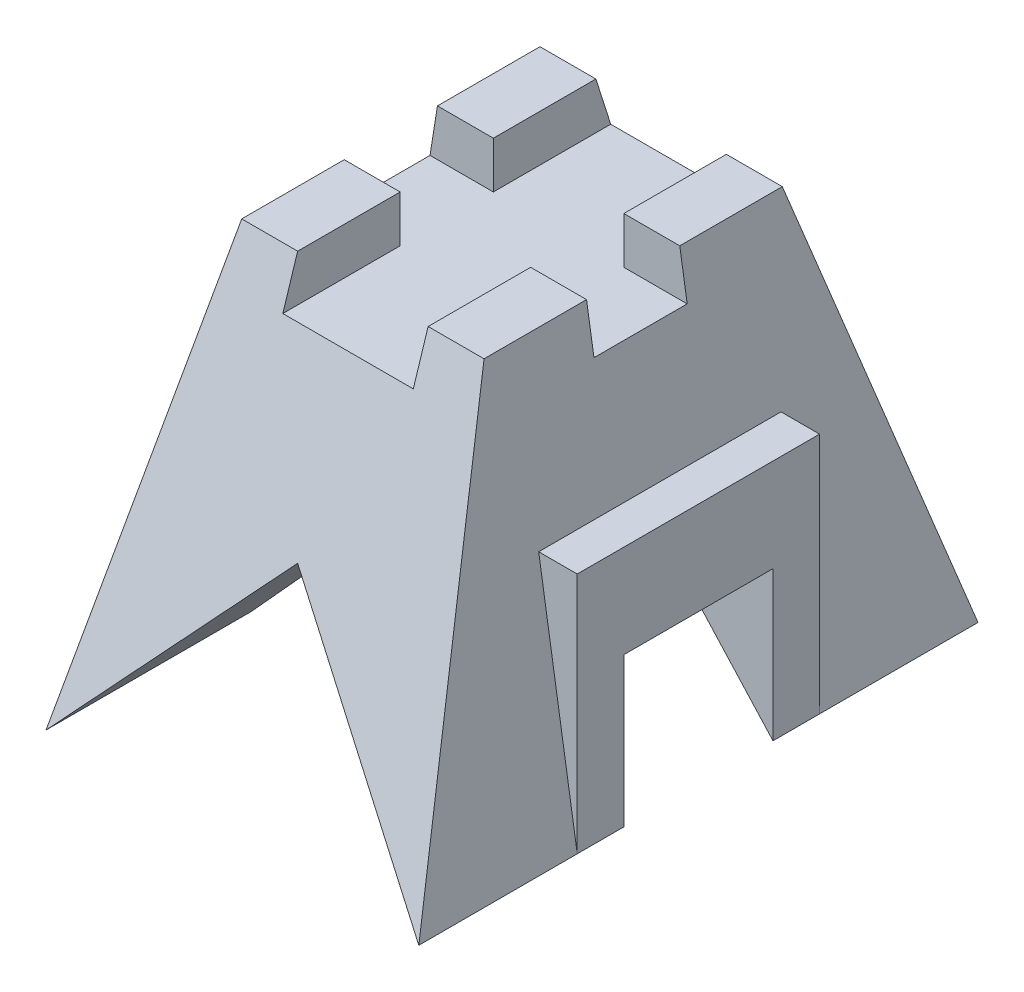
ISO-10303-21;
HEADER;
FILE_DESCRIPTION(('STEP AP214'),'2;1');
FILE_NAME('part.step','',(''),(''),'','','');
FILE_SCHEMA(('AUTOMOTIVE_DESIGN { 1 0 10303 214 1 1 1 1 }'));
ENDSEC;
DATA;
#1=APPLICATION_CONTEXT('core data for automotive mechanical design processes');
#2=APPLICATION_PROTOCOL_DEFINITION('international standard','automotive_design',2000,#1);
#3=PRODUCT_CONTEXT('',#1,'mechanical');
#4=PRODUCT('Part','Part','',(#3));
#5=PRODUCT_RELATED_PRODUCT_CATEGORY('part','',(#4));
#6=PRODUCT_DEFINITION_FORMATION('','',#4);
#7=PRODUCT_DEFINITION_CONTEXT('part definition',#1,'design');
#8=PRODUCT_DEFINITION('design','',#6,#7);
#9=PRODUCT_DEFINITION_SHAPE('','',#8);
#10=(LENGTH_UNIT() NAMED_UNIT(*) SI_UNIT(.MILLI.,.METRE.));
#11=(NAMED_UNIT(*) PLANE_ANGLE_UNIT() SI_UNIT($,.RADIAN.));
#12=(NAMED_UNIT(*) SI_UNIT($,.STERADIAN.) SOLID_ANGLE_UNIT());
#13=UNCERTAINTY_MEASURE_WITH_UNIT(LENGTH_MEASURE(1.E-05),#10,'distance_accuracy_value','');
#14=(GEOMETRIC_REPRESENTATION_CONTEXT(3) GLOBAL_UNCERTAINTY_ASSIGNED_CONTEXT((#13)) GLOBAL_UNIT_ASSIGNED_CONTEXT((#10,
#11,#12)) REPRESENTATION_CONTEXT('',''));
#15=CARTESIAN_POINT('',(0.,0.,0.));
#16=DIRECTION('',(0.,0.,1.));
#17=DIRECTION('',(1.,0.,0.));
#18=AXIS2_PLACEMENT_3D('',#15,#16,#17);
#19=CARTESIAN_POINT('',(100.,0.,65.));
#20=DIRECTION('',(-1.,0.,0.));
#21=DIRECTION('',(0.,0.,1.));
#22=AXIS2_PLACEMENT_3D('',#19,#20,#21);
#23=PLANE('',#22);
#24=DIRECTION('',(0.,-1.,0.));
#25=VECTOR('',#24,1.);
#26=CARTESIAN_POINT('',(100.,0.,40.));
#27=LINE('',#26,#25);
#28=CARTESIAN_POINT('',(100.,80.,40.));
#29=VERTEX_POINT('',#28);
#30=CARTESIAN_POINT('',(100.,0.,40.));
#31=VERTEX_POINT('',#30);
#32=EDGE_CURVE('E103',#29,#31,#27,.T.);
#33=ORIENTED_EDGE('',*,*,#32,.F.);
#34=DIRECTION('',(0.,0.,1.));
#35=VECTOR('',#34,1.);
#36=CARTESIAN_POINT('',(100.,80.,40.));
#37=LINE('',#36,#35);
#38=CARTESIAN_POINT('',(100.,80.,-40.));
#39=VERTEX_POINT('',#38);
#40=EDGE_CURVE('E99',#39,#29,#37,.T.);
#41=ORIENTED_EDGE('',*,*,#40,.F.);
#42=DIRECTION('',(0.,1.,0.));
#43=VECTOR('',#42,1.);
#44=CARTESIAN_POINT('',(100.,0.,-40.));
#45=LINE('',#44,#43);
#46=CARTESIAN_POINT('',(100.,0.,-40.));
#47=VERTEX_POINT('',#46);
#48=EDGE_CURVE('E89',#47,#39,#45,.T.);
#49=ORIENTED_EDGE('',*,*,#48,.F.);
#50=DIRECTION('',(0.,0.,1.));
#51=VECTOR('',#50,1.);
#52=CARTESIAN_POINT('',(100.,0.,65.));
#53=LINE('',#52,#51);
#54=CARTESIAN_POINT('',(100.,0.,-65.));
#55=VERTEX_POINT('',#54);
#56=EDGE_CURVE('E46',#47,#55,#53,.F.);
#57=ORIENTED_EDGE('',*,*,#56,.T.);
#58=DIRECTION('',(0.,1.,0.));
#59=VECTOR('',#58,1.);
#60=CARTESIAN_POINT('',(100.,0.,-65.));
#61=LINE('',#60,#59);
#62=CARTESIAN_POINT('',(100.,130.,-65.));
#63=VERTEX_POINT('',#62);
#64=EDGE_CURVE('E260',#55,#63,#61,.T.);
#65=ORIENTED_EDGE('',*,*,#64,.T.);
#66=DIRECTION('',(0.,0.,-1.));
#67=VECTOR('',#66,1.);
#68=CARTESIAN_POINT('',(100.,130.,65.));
#69=LINE('',#68,#67);
#70=CARTESIAN_POINT('',(100.,130.,65.));
#71=VERTEX_POINT('',#70);
#72=EDGE_CURVE('E107',#71,#63,#69,.T.);
#73=ORIENTED_EDGE('',*,*,#72,.F.);
#74=DIRECTION('',(0.,1.,0.));
#75=VECTOR('',#74,1.);
#76=CARTESIAN_POINT('',(100.,0.,65.));
#77=LINE('',#76,#75);
#78=CARTESIAN_POINT('',(100.,0.,65.));
#79=VERTEX_POINT('',#78);
#80=EDGE_CURVE('E249',#79,#71,#77,.T.);
#81=ORIENTED_EDGE('',*,*,#80,.F.);
#82=DIRECTION('',(0.,0.,1.));
#83=VECTOR('',#82,1.);
#84=CARTESIAN_POINT('',(100.,0.,65.));
#85=LINE('',#84,#83);
#86=EDGE_CURVE('E108',#79,#31,#85,.F.);
#87=ORIENTED_EDGE('',*,*,#86,.T.);
#88=EDGE_LOOP('',(#33,#41,#49,#57,#65,#73,#81,#87));
#89=FACE_BOUND('',#88,.T.);
#90=ADVANCED_FACE('F45',(#89),#23,.F.);
#91=CARTESIAN_POINT('',(-100.,0.,65.));
#92=DIRECTION('',(-1.,0.,0.));
#93=DIRECTION('',(0.,0.,1.));
#94=AXIS2_PLACEMENT_3D('',#91,#92,#93);
#95=PLANE('',#94);
#96=DIRECTION('',(0.,0.,1.));
#97=VECTOR('',#96,1.);
#98=CARTESIAN_POINT('',(-100.,80.,40.));
#99=LINE('',#98,#97);
#100=CARTESIAN_POINT('',(-100.,80.,-40.));
#101=VERTEX_POINT('',#100);
#102=CARTESIAN_POINT('',(-100.,80.,40.));
#103=VERTEX_POINT('',#102);
#104=EDGE_CURVE('E781',#101,#103,#99,.T.);
#105=ORIENTED_EDGE('',*,*,#104,.T.);
#106=DIRECTION('',(0.,-1.,0.));
#107=VECTOR('',#106,1.);
#108=CARTESIAN_POINT('',(-100.,0.,40.));
#109=LINE('',#108,#107);
#110=CARTESIAN_POINT('',(-100.,0.,40.));
#111=VERTEX_POINT('',#110);
#112=EDGE_CURVE('E265',#103,#111,#109,.T.);
#113=ORIENTED_EDGE('',*,*,#112,.T.);
#114=DIRECTION('',(0.,0.,-1.));
#115=VECTOR('',#114,1.);
#116=CARTESIAN_POINT('',(-100.,0.,65.));
#117=LINE('',#116,#115);
#118=CARTESIAN_POINT('',(-100.,0.,65.));
#119=VERTEX_POINT('',#118);
#120=EDGE_CURVE('E393',#119,#111,#117,.T.);
#121=ORIENTED_EDGE('',*,*,#120,.F.);
#122=DIRECTION('',(0.,1.,0.));
#123=VECTOR('',#122,1.);
#124=CARTESIAN_POINT('',(-100.,0.,65.));
#125=LINE('',#124,#123);
#126=CARTESIAN_POINT('',(-100.,130.,65.));
#127=VERTEX_POINT('',#126);
#128=EDGE_CURVE('E378',#119,#127,#125,.T.);
#129=ORIENTED_EDGE('',*,*,#128,.T.);
#130=DIRECTION('',(0.,0.,-1.));
#131=VECTOR('',#130,1.);
#132=CARTESIAN_POINT('',(-100.,130.,65.));
#133=LINE('',#132,#131);
#134=CARTESIAN_POINT('',(-100.,130.,-65.));
#135=VERTEX_POINT('',#134);
#136=EDGE_CURVE('E399',#127,#135,#133,.T.);
#137=ORIENTED_EDGE('',*,*,#136,.T.);
#138=DIRECTION('',(0.,1.,0.));
#139=VECTOR('',#138,1.);
#140=CARTESIAN_POINT('',(-100.,0.,-65.));
#141=LINE('',#140,#139);
#142=CARTESIAN_POINT('',(-100.,0.,-65.));
#143=VERTEX_POINT('',#142);
#144=EDGE_CURVE('E409',#143,#135,#141,.T.);
#145=ORIENTED_EDGE('',*,*,#144,.F.);
#146=CARTESIAN_POINT('',(-100.,0.,-40.));
#147=VERTEX_POINT('',#146);
#148=EDGE_CURVE('E388',#147,#143,#117,.T.);
#149=ORIENTED_EDGE('',*,*,#148,.F.);
#150=DIRECTION('',(0.,1.,0.));
#151=VECTOR('',#150,1.);
#152=CARTESIAN_POINT('',(-100.,0.,-40.));
#153=LINE('',#152,#151);
#154=EDGE_CURVE('E788',#147,#101,#153,.T.);
#155=ORIENTED_EDGE('',*,*,#154,.T.);
#156=EDGE_LOOP('',(#105,#113,#121,#129,#137,#145,#149,#155));
#157=FACE_BOUND('',#156,.T.);
#158=ADVANCED_FACE('F398',(#157),#95,.T.);
#159=CARTESIAN_POINT('',(65.,220.,-150.));
#160=DIRECTION('',(0.987580306335114,0.157115048735132,0.));
#161=DIRECTION('',(-0.157115048735132,0.987580306335114,0.));
#162=AXIS2_PLACEMENT_3D('',#159,#160,#161);
#163=PLANE('',#162);
#164=DIRECTION('',(0.,0.,-1.));
#165=VECTOR('',#164,1.);
#166=CARTESIAN_POINT('',(79.3181818181818,130.,65.));
#167=LINE('',#166,#165);
#168=CARTESIAN_POINT('',(79.3181818181818,130.,65.));
#169=VERTEX_POINT('',#168);
#170=CARTESIAN_POINT('',(79.3181818181818,130.,-65.));
#171=VERTEX_POINT('',#170);
#172=EDGE_CURVE('E113',#169,#171,#167,.T.);
#173=ORIENTED_EDGE('',*,*,#172,.T.);
#174=DIRECTION('',(0.157115048735132,-0.987580306335114,0.));
#175=VECTOR('',#174,1.);
#176=CARTESIAN_POINT('',(79.3181818181818,130.,-65.));
#177=LINE('',#176,#175);
#178=EDGE_CURVE('E256',#171,#55,#177,.T.);
#179=ORIENTED_EDGE('',*,*,#178,.T.);
#180=DIRECTION('',(0.,0.,-1.));
#181=VECTOR('',#180,1.);
#182=CARTESIAN_POINT('',(100.,0.,-150.));
#183=LINE('',#182,#181);
#184=CARTESIAN_POINT('',(100.,0.,-150.));
#185=VERTEX_POINT('',#184);
#186=EDGE_CURVE('E110',#55,#185,#183,.T.);
#187=ORIENTED_EDGE('',*,*,#186,.T.);
#188=DIRECTION('',(-0.149889153602658,0.942160394073851,0.299778307205316));
#189=VECTOR('',#188,1.);
#190=CARTESIAN_POINT('',(65.7863365428702,215.057313159101,-81.5726730857405));
#191=LINE('',#190,#189);
#192=CARTESIAN_POINT('',(65.,220.,-80.));
#193=VERTEX_POINT('',#192);
#194=EDGE_CURVE('E168',#185,#193,#191,.T.);
#195=ORIENTED_EDGE('',*,*,#194,.T.);
#196=DIRECTION('',(0.,0.,1.));
#197=VECTOR('',#196,1.);
#198=CARTESIAN_POINT('',(65.,220.,-150.));
#199=LINE('',#198,#197);
#200=CARTESIAN_POINT('',(65.,220.,-25.));
#201=VERTEX_POINT('',#200);
#202=EDGE_CURVE('E153',#193,#201,#199,.T.);
#203=ORIENTED_EDGE('',*,*,#202,.T.);
#204=DIRECTION('',(0.157115048735132,-0.987580306335114,0.));
#205=VECTOR('',#204,1.);
#206=CARTESIAN_POINT('',(65.8639798488665,214.569269521411,-25.));
#207=LINE('',#206,#205);
#208=CARTESIAN_POINT('',(68.9772727272727,195.,-25.));
#209=VERTEX_POINT('',#208);
#210=EDGE_CURVE('E161',#201,#209,#207,.T.);
#211=ORIENTED_EDGE('',*,*,#210,.T.);
#212=DIRECTION('',(0.,0.,1.));
#213=VECTOR('',#212,1.);
#214=CARTESIAN_POINT('',(68.9772727272727,195.,25.));
#215=LINE('',#214,#213);
#216=CARTESIAN_POINT('',(68.9772727272727,195.,25.));
#217=VERTEX_POINT('',#216);
#218=EDGE_CURVE('E157',#209,#217,#215,.T.);
#219=ORIENTED_EDGE('',*,*,#218,.T.);
#220=DIRECTION('',(-0.157115048735132,0.987580306335114,0.));
#221=VECTOR('',#220,1.);
#222=CARTESIAN_POINT('',(65.8639798488665,214.569269521411,25.));
#223=LINE('',#222,#221);
#224=CARTESIAN_POINT('',(65.,220.,25.));
#225=VERTEX_POINT('',#224);
#226=EDGE_CURVE('E160',#217,#225,#223,.T.);
#227=ORIENTED_EDGE('',*,*,#226,.T.);
#228=CARTESIAN_POINT('',(65.,220.,80.));
#229=VERTEX_POINT('',#228);
#230=EDGE_CURVE('E135',#225,#229,#199,.T.);
#231=ORIENTED_EDGE('',*,*,#230,.T.);
#232=DIRECTION('',(0.149889153602658,-0.942160394073851,0.299778307205316));
#233=VECTOR('',#232,1.);
#234=CARTESIAN_POINT('',(100.,0.,150.));
#235=LINE('',#234,#233);
#236=CARTESIAN_POINT('',(100.,0.,150.));
#237=VERTEX_POINT('',#236);
#238=EDGE_CURVE('E231',#229,#237,#235,.T.);
#239=ORIENTED_EDGE('',*,*,#238,.T.);
#240=EDGE_CURVE('E201',#237,#79,#183,.T.);
#241=ORIENTED_EDGE('',*,*,#240,.T.);
#242=DIRECTION('',(0.157115048735132,-0.987580306335114,0.));
#243=VECTOR('',#242,1.);
#244=CARTESIAN_POINT('',(79.3181818181818,130.,65.));
#245=LINE('',#244,#243);
#246=EDGE_CURVE('E254',#169,#79,#245,.T.);
#247=ORIENTED_EDGE('',*,*,#246,.F.);
#248=EDGE_LOOP('',(#173,#179,#187,#195,#203,#211,#219,#227,#231,#239,#241,#247));
#249=FACE_BOUND('',#248,.T.);
#250=ADVANCED_FACE('F288',(#249),#163,.T.);
#251=CARTESIAN_POINT('',(100.,220.,-25.));
#252=DIRECTION('',(0.,-1.,0.));
#253=DIRECTION('',(0.,0.,-1.));
#254=AXIS2_PLACEMENT_3D('',#251,#252,#253);
#255=PLANE('',#254);
#256=DIRECTION('',(0.,0.,1.));
#257=VECTOR('',#256,1.);
#258=CARTESIAN_POINT('',(-35.,220.,-150.));
#259=LINE('',#258,#257);
#260=CARTESIAN_POINT('',(-35.,220.,-80.));
#261=VERTEX_POINT('',#260);
#262=CARTESIAN_POINT('',(-35.,220.,-25.));
#263=VERTEX_POINT('',#262);
#264=EDGE_CURVE('E136',#261,#263,#259,.T.);
#265=ORIENTED_EDGE('',*,*,#264,.F.);
#266=DIRECTION('',(-1.,0.,0.));
#267=VECTOR('',#266,1.);
#268=CARTESIAN_POINT('',(100.,220.,-80.));
#269=LINE('',#268,#267);
#270=CARTESIAN_POINT('',(-65.,220.,-80.));
#271=VERTEX_POINT('',#270);
#272=EDGE_CURVE('E230',#261,#271,#269,.T.);
#273=ORIENTED_EDGE('',*,*,#272,.T.);
#274=DIRECTION('',(0.,0.,1.));
#275=VECTOR('',#274,1.);
#276=CARTESIAN_POINT('',(-65.,220.,-150.));
#277=LINE('',#276,#275);
#278=CARTESIAN_POINT('',(-65.,220.,-25.));
#279=VERTEX_POINT('',#278);
#280=EDGE_CURVE('E140',#271,#279,#277,.T.);
#281=ORIENTED_EDGE('',*,*,#280,.T.);
#282=DIRECTION('',(-1.,0.,0.));
#283=VECTOR('',#282,1.);
#284=CARTESIAN_POINT('',(100.,220.,-25.));
#285=LINE('',#284,#283);
#286=EDGE_CURVE('E222',#263,#279,#285,.T.);
#287=ORIENTED_EDGE('',*,*,#286,.F.);
#288=EDGE_LOOP('',(#265,#273,#281,#287));
#289=FACE_BOUND('',#288,.T.);
#290=ADVANCED_FACE('F445',(#289),#255,.F.);
#291=ORIENTED_EDGE('',*,*,#202,.F.);
#292=CARTESIAN_POINT('',(35.,220.,-80.));
#293=VERTEX_POINT('',#292);
#294=EDGE_CURVE('E235',#193,#293,#269,.T.);
#295=ORIENTED_EDGE('',*,*,#294,.T.);
#296=DIRECTION('',(0.,0.,1.));
#297=VECTOR('',#296,1.);
#298=CARTESIAN_POINT('',(35.,220.,-150.));
#299=LINE('',#298,#297);
#300=CARTESIAN_POINT('',(35.,220.,-25.));
#301=VERTEX_POINT('',#300);
#302=EDGE_CURVE('E148',#293,#301,#299,.T.);
#303=ORIENTED_EDGE('',*,*,#302,.T.);
#304=EDGE_CURVE('E226',#201,#301,#285,.T.);
#305=ORIENTED_EDGE('',*,*,#304,.F.);
#306=EDGE_LOOP('',(#291,#295,#303,#305));
#307=FACE_BOUND('',#306,.T.);
#308=ADVANCED_FACE('F542',(#307),#255,.F.);
#309=CARTESIAN_POINT('',(100.,220.,80.));
#310=DIRECTION('',(0.,-1.,0.));
#311=DIRECTION('',(0.,0.,-1.));
#312=AXIS2_PLACEMENT_3D('',#309,#310,#311);
#313=PLANE('',#312);
#314=CARTESIAN_POINT('',(-35.,220.,25.));
#315=VERTEX_POINT('',#314);
#316=CARTESIAN_POINT('',(-35.,220.,79.9999999999999));
#317=VERTEX_POINT('',#316);
#318=EDGE_CURVE('E139',#315,#317,#259,.T.);
#319=ORIENTED_EDGE('',*,*,#318,.F.);
#320=DIRECTION('',(-1.,0.,0.));
#321=VECTOR('',#320,1.);
#322=CARTESIAN_POINT('',(100.,220.,25.));
#323=LINE('',#322,#321);
#324=CARTESIAN_POINT('',(-65.,220.,25.));
#325=VERTEX_POINT('',#324);
#326=EDGE_CURVE('E214',#315,#325,#323,.T.);
#327=ORIENTED_EDGE('',*,*,#326,.T.);
#328=CARTESIAN_POINT('',(-65.,220.,80.));
#329=VERTEX_POINT('',#328);
#330=EDGE_CURVE('E133',#325,#329,#277,.T.);
#331=ORIENTED_EDGE('',*,*,#330,.T.);
#332=DIRECTION('',(-1.,0.,0.));
#333=VECTOR('',#332,1.);
#334=CARTESIAN_POINT('',(100.,220.,80.));
#335=LINE('',#334,#333);
#336=EDGE_CURVE('E207',#317,#329,#335,.T.);
#337=ORIENTED_EDGE('',*,*,#336,.F.);
#338=EDGE_LOOP('',(#319,#327,#331,#337));
#339=FACE_BOUND('',#338,.T.);
#340=ADVANCED_FACE('F417',(#339),#313,.F.);
#341=ORIENTED_EDGE('',*,*,#230,.F.);
#342=CARTESIAN_POINT('',(35.,220.,25.));
#343=VERTEX_POINT('',#342);
#344=EDGE_CURVE('E219',#225,#343,#323,.T.);
#345=ORIENTED_EDGE('',*,*,#344,.T.);
#346=CARTESIAN_POINT('',(35.,220.,80.));
#347=VERTEX_POINT('',#346);
#348=EDGE_CURVE('E154',#343,#347,#299,.T.);
#349=ORIENTED_EDGE('',*,*,#348,.T.);
#350=EDGE_CURVE('E215',#229,#347,#335,.T.);
#351=ORIENTED_EDGE('',*,*,#350,.F.);
#352=EDGE_LOOP('',(#341,#345,#349,#351));
#353=FACE_BOUND('',#352,.T.);
#354=ADVANCED_FACE('F543',(#353),#313,.F.);
#355=CARTESIAN_POINT('',(100.,220.,-80.));
#356=DIRECTION('',(0.,-0.303203657276947,0.952925780013262));
#357=DIRECTION('',(0.,-0.952925780013262,-0.303203657276947));
#358=AXIS2_PLACEMENT_3D('',#355,#356,#357);
#359=PLANE('',#358);
#360=DIRECTION('',(-0.654770604471651,0.720247664918816,0.229169711565078));
#361=VECTOR('',#360,1.);
#362=CARTESIAN_POINT('',(-14.2550911039657,125.680600214362,-110.010718113612));
#363=LINE('',#362,#361);
#364=CARTESIAN_POINT('',(0.,110.,-115.));
#365=VERTEX_POINT('',#364);
#366=EDGE_CURVE('E130',#185,#365,#363,.T.);
#367=ORIENTED_EDGE('',*,*,#366,.T.);
#368=DIRECTION('',(-0.654770604471651,-0.720247664918816,-0.229169711565078));
#369=VECTOR('',#368,1.);
#370=CARTESIAN_POINT('',(100.,220.,-80.));
#371=LINE('',#370,#369);
#372=CARTESIAN_POINT('',(-100.,0.,-150.));
#373=VERTEX_POINT('',#372);
#374=EDGE_CURVE('E128',#365,#373,#371,.T.);
#375=ORIENTED_EDGE('',*,*,#374,.T.);
#376=DIRECTION('',(-0.149889153602658,-0.942160394073851,-0.299778307205316));
#377=VECTOR('',#376,1.);
#378=CARTESIAN_POINT('',(-61.292984869326,243.301237964237,-72.585969738652));
#379=LINE('',#378,#377);
#380=EDGE_CURVE('E198',#271,#373,#379,.T.);
#381=ORIENTED_EDGE('',*,*,#380,.F.);
#382=ORIENTED_EDGE('',*,*,#272,.F.);
#383=DIRECTION('',(0.,0.952925780013262,0.303203657276947));
#384=VECTOR('',#383,1.);
#385=CARTESIAN_POINT('',(-35.,220.,-80.));
#386=LINE('',#385,#384);
#387=CARTESIAN_POINT('',(-35.,195.,-87.9545454545455));
#388=VERTEX_POINT('',#387);
#389=EDGE_CURVE('E190',#388,#261,#386,.T.);
#390=ORIENTED_EDGE('',*,*,#389,.F.);
#391=DIRECTION('',(-1.,0.,0.));
#392=VECTOR('',#391,1.);
#393=CARTESIAN_POINT('',(100.,195.,-87.9545454545455));
#394=LINE('',#393,#392);
#395=CARTESIAN_POINT('',(35.,195.,-87.9545454545455));
#396=VERTEX_POINT('',#395);
#397=EDGE_CURVE('E178',#396,#388,#394,.T.);
#398=ORIENTED_EDGE('',*,*,#397,.F.);
#399=DIRECTION('',(0.,-0.952925780013262,-0.303203657276947));
#400=VECTOR('',#399,1.);
#401=CARTESIAN_POINT('',(35.,220.,-80.));
#402=LINE('',#401,#400);
#403=EDGE_CURVE('E174',#293,#396,#402,.T.);
#404=ORIENTED_EDGE('',*,*,#403,.F.);
#405=ORIENTED_EDGE('',*,*,#294,.F.);
#406=ORIENTED_EDGE('',*,*,#194,.F.);
#407=EDGE_LOOP('',(#367,#375,#381,#382,#390,#398,#404,#405,#406));
#408=FACE_BOUND('',#407,.T.);
#409=ADVANCED_FACE('F42',(#408),#359,.F.);
#410=CARTESIAN_POINT('',(100.,220.,-25.));
#411=DIRECTION('',(0.,0.,-1.));
#412=DIRECTION('',(0.,1.,0.));
#413=AXIS2_PLACEMENT_3D('',#410,#411,#412);
#414=PLANE('',#413);
#415=DIRECTION('',(0.157115048735132,0.987580306335114,0.));
#416=VECTOR('',#415,1.);
#417=CARTESIAN_POINT('',(-60.926952141058,245.60201511335,-25.));
#418=LINE('',#417,#416);
#419=CARTESIAN_POINT('',(-68.9772727272727,195.,-25.));
#420=VERTEX_POINT('',#419);
#421=EDGE_CURVE('E199',#420,#279,#418,.T.);
#422=ORIENTED_EDGE('',*,*,#421,.F.);
#423=DIRECTION('',(-1.,0.,0.));
#424=VECTOR('',#423,1.);
#425=CARTESIAN_POINT('',(100.,195.,-25.));
#426=LINE('',#425,#424);
#427=CARTESIAN_POINT('',(-35.,195.,-25.));
#428=VERTEX_POINT('',#427);
#429=EDGE_CURVE('E223',#428,#420,#426,.T.);
#430=ORIENTED_EDGE('',*,*,#429,.F.);
#431=DIRECTION('',(0.,-1.,0.));
#432=VECTOR('',#431,1.);
#433=CARTESIAN_POINT('',(-35.,220.,-25.));
#434=LINE('',#433,#432);
#435=EDGE_CURVE('E183',#263,#428,#434,.T.);
#436=ORIENTED_EDGE('',*,*,#435,.F.);
#437=ORIENTED_EDGE('',*,*,#286,.T.);
#438=EDGE_LOOP('',(#422,#430,#436,#437));
#439=FACE_BOUND('',#438,.T.);
#440=ADVANCED_FACE('F436',(#439),#414,.F.);
#441=DIRECTION('',(0.,1.,0.));
#442=VECTOR('',#441,1.);
#443=CARTESIAN_POINT('',(35.,220.,-25.));
#444=LINE('',#443,#442);
#445=CARTESIAN_POINT('',(35.,195.,-25.));
#446=VERTEX_POINT('',#445);
#447=EDGE_CURVE('E175',#446,#301,#444,.T.);
#448=ORIENTED_EDGE('',*,*,#447,.F.);
#449=EDGE_CURVE('E224',#209,#446,#426,.T.);
#450=ORIENTED_EDGE('',*,*,#449,.F.);
#451=ORIENTED_EDGE('',*,*,#210,.F.);
#452=ORIENTED_EDGE('',*,*,#304,.T.);
#453=EDGE_LOOP('',(#448,#450,#451,#452));
#454=FACE_BOUND('',#453,.T.);
#455=ADVANCED_FACE('F547',(#454),#414,.F.);
#456=CARTESIAN_POINT('',(100.,195.,25.));
#457=DIRECTION('',(0.,-1.,0.));
#458=DIRECTION('',(0.,0.,-1.));
#459=AXIS2_PLACEMENT_3D('',#456,#457,#458);
#460=PLANE('',#459);
#461=ORIENTED_EDGE('',*,*,#449,.T.);
#462=DIRECTION('',(0.,0.,1.));
#463=VECTOR('',#462,1.);
#464=CARTESIAN_POINT('',(35.,195.,-150.));
#465=LINE('',#464,#463);
#466=EDGE_CURVE('E147',#396,#446,#465,.T.);
#467=ORIENTED_EDGE('',*,*,#466,.F.);
#468=ORIENTED_EDGE('',*,*,#397,.T.);
#469=DIRECTION('',(0.,0.,1.));
#470=VECTOR('',#469,1.);
#471=CARTESIAN_POINT('',(-35.,195.,-150.));
#472=LINE('',#471,#470);
#473=EDGE_CURVE('E145',#388,#428,#472,.T.);
#474=ORIENTED_EDGE('',*,*,#473,.T.);
#475=ORIENTED_EDGE('',*,*,#429,.T.);
#476=DIRECTION('',(0.,0.,-1.));
#477=VECTOR('',#476,1.);
#478=CARTESIAN_POINT('',(-68.9772727272727,195.,25.));
#479=LINE('',#478,#477);
#480=CARTESIAN_POINT('',(-68.9772727272727,195.,25.));
#481=VERTEX_POINT('',#480);
#482=EDGE_CURVE('E194',#481,#420,#479,.T.);
#483=ORIENTED_EDGE('',*,*,#482,.F.);
#484=DIRECTION('',(-1.,0.,0.));
#485=VECTOR('',#484,1.);
#486=CARTESIAN_POINT('',(100.,195.,25.));
#487=LINE('',#486,#485);
#488=CARTESIAN_POINT('',(-35.,195.,25.));
#489=VERTEX_POINT('',#488);
#490=EDGE_CURVE('E216',#489,#481,#487,.T.);
#491=ORIENTED_EDGE('',*,*,#490,.F.);
#492=CARTESIAN_POINT('',(-35.,195.,87.9545454545455));
#493=VERTEX_POINT('',#492);
#494=EDGE_CURVE('E141',#489,#493,#472,.T.);
#495=ORIENTED_EDGE('',*,*,#494,.T.);
#496=DIRECTION('',(1.,0.,0.));
#497=VECTOR('',#496,1.);
#498=CARTESIAN_POINT('',(100.,195.,87.9545454545455));
#499=LINE('',#498,#497);
#500=CARTESIAN_POINT('',(35.,195.,87.9545454545455));
#501=VERTEX_POINT('',#500);
#502=EDGE_CURVE('E237',#493,#501,#499,.T.);
#503=ORIENTED_EDGE('',*,*,#502,.T.);
#504=CARTESIAN_POINT('',(35.,195.,25.));
#505=VERTEX_POINT('',#504);
#506=EDGE_CURVE('E150',#505,#501,#465,.T.);
#507=ORIENTED_EDGE('',*,*,#506,.F.);
#508=EDGE_CURVE('E217',#217,#505,#487,.T.);
#509=ORIENTED_EDGE('',*,*,#508,.F.);
#510=ORIENTED_EDGE('',*,*,#218,.F.);
#511=EDGE_LOOP('',(#461,#467,#468,#474,#475,#483,#491,#495,#503,#507,#509,#510));
#512=FACE_BOUND('',#511,.T.);
#513=ADVANCED_FACE('F427',(#512),#460,.F.);
#514=CARTESIAN_POINT('',(100.,220.,25.));
#515=DIRECTION('',(0.,0.,1.));
#516=DIRECTION('',(0.,-1.,0.));
#517=AXIS2_PLACEMENT_3D('',#514,#515,#516);
#518=PLANE('',#517);
#519=DIRECTION('',(-0.157115048735132,-0.987580306335114,0.));
#520=VECTOR('',#519,1.);
#521=CARTESIAN_POINT('',(-60.926952141058,245.60201511335,25.));
#522=LINE('',#521,#520);
#523=EDGE_CURVE('E188',#325,#481,#522,.T.);
#524=ORIENTED_EDGE('',*,*,#523,.F.);
#525=ORIENTED_EDGE('',*,*,#326,.F.);
#526=DIRECTION('',(0.,1.,0.));
#527=VECTOR('',#526,1.);
#528=CARTESIAN_POINT('',(-35.,220.,25.));
#529=LINE('',#528,#527);
#530=EDGE_CURVE('E181',#489,#315,#529,.T.);
#531=ORIENTED_EDGE('',*,*,#530,.F.);
#532=ORIENTED_EDGE('',*,*,#490,.T.);
#533=EDGE_LOOP('',(#524,#525,#531,#532));
#534=FACE_BOUND('',#533,.T.);
#535=ADVANCED_FACE('F425',(#534),#518,.F.);
#536=DIRECTION('',(0.,-1.,0.));
#537=VECTOR('',#536,1.);
#538=CARTESIAN_POINT('',(35.,220.,25.));
#539=LINE('',#538,#537);
#540=EDGE_CURVE('E169',#343,#505,#539,.T.);
#541=ORIENTED_EDGE('',*,*,#540,.F.);
#542=ORIENTED_EDGE('',*,*,#344,.F.);
#543=ORIENTED_EDGE('',*,*,#226,.F.);
#544=ORIENTED_EDGE('',*,*,#508,.T.);
#545=EDGE_LOOP('',(#541,#542,#543,#544));
#546=FACE_BOUND('',#545,.T.);
#547=ADVANCED_FACE('F544',(#546),#518,.F.);
#548=CARTESIAN_POINT('',(100.,0.,150.));
#549=DIRECTION('',(0.,-0.303203657276947,-0.952925780013262));
#550=DIRECTION('',(0.,0.952925780013262,-0.303203657276947));
#551=AXIS2_PLACEMENT_3D('',#548,#549,#550);
#552=PLANE('',#551);
#553=DIRECTION('',(0.149889153602658,0.942160394073851,-0.299778307205316));
#554=VECTOR('',#553,1.);
#555=CARTESIAN_POINT('',(-95.5066483264557,28.2439248051352,141.013296652912));
#556=LINE('',#555,#554);
#557=CARTESIAN_POINT('',(-100.,0.,150.));
#558=VERTEX_POINT('',#557);
#559=EDGE_CURVE('E244',#558,#329,#556,.T.);
#560=ORIENTED_EDGE('',*,*,#559,.F.);
#561=DIRECTION('',(0.654770604471651,0.720247664918816,-0.229169711565078));
#562=VECTOR('',#561,1.);
#563=CARTESIAN_POINT('',(-14.2550911039657,94.3193997856377,119.989281886388));
#564=LINE('',#563,#562);
#565=CARTESIAN_POINT('',(0.,110.,115.));
#566=VERTEX_POINT('',#565);
#567=EDGE_CURVE('E12',#558,#566,#564,.T.);
#568=ORIENTED_EDGE('',*,*,#567,.T.);
#569=DIRECTION('',(0.654770604471651,-0.720247664918816,0.229169711565078));
#570=VECTOR('',#569,1.);
#571=CARTESIAN_POINT('',(100.,0.,150.));
#572=LINE('',#571,#570);
#573=EDGE_CURVE('E55',#566,#237,#572,.T.);
#574=ORIENTED_EDGE('',*,*,#573,.T.);
#575=ORIENTED_EDGE('',*,*,#238,.F.);
#576=ORIENTED_EDGE('',*,*,#350,.T.);
#577=DIRECTION('',(0.,0.952925780013262,-0.303203657276947));
#578=VECTOR('',#577,1.);
#579=CARTESIAN_POINT('',(35.,0.,150.));
#580=LINE('',#579,#578);
#581=EDGE_CURVE('E236',#501,#347,#580,.T.);
#582=ORIENTED_EDGE('',*,*,#581,.F.);
#583=ORIENTED_EDGE('',*,*,#502,.F.);
#584=DIRECTION('',(0.,-0.952925780013262,0.303203657276947));
#585=VECTOR('',#584,1.);
#586=CARTESIAN_POINT('',(-35.,0.,150.));
#587=LINE('',#586,#585);
#588=EDGE_CURVE('E245',#317,#493,#587,.T.);
#589=ORIENTED_EDGE('',*,*,#588,.F.);
#590=ORIENTED_EDGE('',*,*,#336,.T.);
#591=EDGE_LOOP('',(#560,#568,#574,#575,#576,#582,#583,#589,#590));
#592=FACE_BOUND('',#591,.T.);
#593=ADVANCED_FACE('F415',(#592),#552,.F.);
#594=CARTESIAN_POINT('',(35.,220.,-150.));
#595=DIRECTION('',(-1.,0.,0.));
#596=DIRECTION('',(0.,-1.,0.));
#597=AXIS2_PLACEMENT_3D('',#594,#595,#596);
#598=PLANE('',#597);
#599=ORIENTED_EDGE('',*,*,#540,.T.);
#600=ORIENTED_EDGE('',*,*,#506,.T.);
#601=ORIENTED_EDGE('',*,*,#581,.T.);
#602=ORIENTED_EDGE('',*,*,#348,.F.);
#603=EDGE_LOOP('',(#599,#600,#601,#602));
#604=FACE_BOUND('',#603,.T.);
#605=ADVANCED_FACE('F537',(#604),#598,.T.);
#606=CARTESIAN_POINT('',(-35.,220.,-150.));
#607=DIRECTION('',(1.,0.,0.));
#608=DIRECTION('',(0.,1.,0.));
#609=AXIS2_PLACEMENT_3D('',#606,#607,#608);
#610=PLANE('',#609);
#611=ORIENTED_EDGE('',*,*,#530,.T.);
#612=ORIENTED_EDGE('',*,*,#318,.T.);
#613=ORIENTED_EDGE('',*,*,#588,.T.);
#614=ORIENTED_EDGE('',*,*,#494,.F.);
#615=EDGE_LOOP('',(#611,#612,#613,#614));
#616=FACE_BOUND('',#615,.T.);
#617=ADVANCED_FACE('F529',(#616),#610,.T.);
#618=CARTESIAN_POINT('',(-100.,0.,-150.));
#619=DIRECTION('',(-0.987580306335114,0.157115048735132,0.));
#620=DIRECTION('',(-0.157115048735132,-0.987580306335114,0.));
#621=AXIS2_PLACEMENT_3D('',#618,#619,#620);
#622=PLANE('',#621);
#623=DIRECTION('',(-0.157115048735132,-0.987580306335114,0.));
#624=VECTOR('',#623,1.);
#625=CARTESIAN_POINT('',(-79.3181818181818,130.,-65.));
#626=LINE('',#625,#624);
#627=CARTESIAN_POINT('',(-79.3181818181818,130.,-65.));
#628=VERTEX_POINT('',#627);
#629=EDGE_CURVE('E452',#628,#143,#626,.T.);
#630=ORIENTED_EDGE('',*,*,#629,.F.);
#631=DIRECTION('',(0.,0.,-1.));
#632=VECTOR('',#631,1.);
#633=CARTESIAN_POINT('',(-79.3181818181818,130.,65.));
#634=LINE('',#633,#632);
#635=CARTESIAN_POINT('',(-79.3181818181818,130.,65.));
#636=VERTEX_POINT('',#635);
#637=EDGE_CURVE('E261',#636,#628,#634,.T.);
#638=ORIENTED_EDGE('',*,*,#637,.F.);
#639=DIRECTION('',(-0.157115048735132,-0.987580306335114,0.));
#640=VECTOR('',#639,1.);
#641=CARTESIAN_POINT('',(-79.3181818181818,130.,65.));
#642=LINE('',#641,#640);
#643=EDGE_CURVE('E381',#636,#119,#642,.T.);
#644=ORIENTED_EDGE('',*,*,#643,.T.);
#645=DIRECTION('',(0.,0.,-1.));
#646=VECTOR('',#645,1.);
#647=CARTESIAN_POINT('',(-100.,0.,-150.));
#648=LINE('',#647,#646);
#649=EDGE_CURVE('E210',#558,#119,#648,.T.);
#650=ORIENTED_EDGE('',*,*,#649,.F.);
#651=ORIENTED_EDGE('',*,*,#559,.T.);
#652=ORIENTED_EDGE('',*,*,#330,.F.);
#653=ORIENTED_EDGE('',*,*,#523,.T.);
#654=ORIENTED_EDGE('',*,*,#482,.T.);
#655=ORIENTED_EDGE('',*,*,#421,.T.);
#656=ORIENTED_EDGE('',*,*,#280,.F.);
#657=ORIENTED_EDGE('',*,*,#380,.T.);
#658=EDGE_CURVE('E205',#143,#373,#648,.T.);
#659=ORIENTED_EDGE('',*,*,#658,.F.);
#660=EDGE_LOOP('',(#630,#638,#644,#650,#651,#652,#653,#654,#655,#656,#657,#659));
#661=FACE_BOUND('',#660,.T.);
#662=ADVANCED_FACE('F403',(#661),#622,.T.);
#663=ORIENTED_EDGE('',*,*,#389,.T.);
#664=ORIENTED_EDGE('',*,*,#264,.T.);
#665=ORIENTED_EDGE('',*,*,#435,.T.);
#666=ORIENTED_EDGE('',*,*,#473,.F.);
#667=EDGE_LOOP('',(#663,#664,#665,#666));
#668=FACE_BOUND('',#667,.T.);
#669=ADVANCED_FACE('F526',(#668),#610,.T.);
#670=ORIENTED_EDGE('',*,*,#403,.T.);
#671=ORIENTED_EDGE('',*,*,#466,.T.);
#672=ORIENTED_EDGE('',*,*,#447,.T.);
#673=ORIENTED_EDGE('',*,*,#302,.F.);
#674=EDGE_LOOP('',(#670,#671,#672,#673));
#675=FACE_BOUND('',#674,.T.);
#676=ADVANCED_FACE('F523',(#675),#598,.T.);
#677=CARTESIAN_POINT('',(-100.,0.,-150.));
#678=DIRECTION('',(-0.739940073395944,0.672672793996313,0.));
#679=DIRECTION('',(-0.672672793996313,-0.739940073395944,0.));
#680=AXIS2_PLACEMENT_3D('',#677,#678,#679);
#681=PLANE('',#680);
#682=ORIENTED_EDGE('',*,*,#120,.T.);
#683=DIRECTION('',(0.672672793996313,0.739940073395944,0.));
#684=VECTOR('',#683,1.);
#685=CARTESIAN_POINT('',(-100.,0.,40.));
#686=LINE('',#685,#684);
#687=CARTESIAN_POINT('',(-27.2727272727272,80.,40.));
#688=VERTEX_POINT('',#687);
#689=EDGE_CURVE('E277',#111,#688,#686,.T.);
#690=ORIENTED_EDGE('',*,*,#689,.T.);
#691=DIRECTION('',(0.,0.,-1.));
#692=VECTOR('',#691,1.);
#693=CARTESIAN_POINT('',(-27.2727272727272,80.,-150.));
#694=LINE('',#693,#692);
#695=CARTESIAN_POINT('',(-27.2727272727272,80.,-40.));
#696=VERTEX_POINT('',#695);
#697=EDGE_CURVE('E280',#688,#696,#694,.T.);
#698=ORIENTED_EDGE('',*,*,#697,.T.);
#699=DIRECTION('',(-0.672672793996313,-0.739940073395944,0.));
#700=VECTOR('',#699,1.);
#701=CARTESIAN_POINT('',(-100.,0.,-40.));
#702=LINE('',#701,#700);
#703=EDGE_CURVE('E93',#696,#147,#702,.T.);
#704=ORIENTED_EDGE('',*,*,#703,.T.);
#705=ORIENTED_EDGE('',*,*,#148,.T.);
#706=ORIENTED_EDGE('',*,*,#658,.T.);
#707=ORIENTED_EDGE('',*,*,#374,.F.);
#708=DIRECTION('',(0.,0.,1.));
#709=VECTOR('',#708,1.);
#710=CARTESIAN_POINT('',(0.,110.,-150.));
#711=LINE('',#710,#709);
#712=EDGE_CURVE('E111',#365,#566,#711,.T.);
#713=ORIENTED_EDGE('',*,*,#712,.T.);
#714=ORIENTED_EDGE('',*,*,#567,.F.);
#715=ORIENTED_EDGE('',*,*,#649,.T.);
#716=EDGE_LOOP('',(#682,#690,#698,#704,#705,#706,#707,#713,#714,#715));
#717=FACE_BOUND('',#716,.T.);
#718=ADVANCED_FACE('F408',(#717),#681,.F.);
#719=CARTESIAN_POINT('',(0.,110.,-150.));
#720=DIRECTION('',(0.739940073395944,0.672672793996313,0.));
#721=DIRECTION('',(-0.672672793996313,0.739940073395944,0.));
#722=AXIS2_PLACEMENT_3D('',#719,#720,#721);
#723=PLANE('',#722);
#724=DIRECTION('',(0.,0.,1.));
#725=VECTOR('',#724,1.);
#726=CARTESIAN_POINT('',(27.2727272727272,80.,-150.));
#727=LINE('',#726,#725);
#728=CARTESIAN_POINT('',(27.2727272727272,80.,-40.));
#729=VERTEX_POINT('',#728);
#730=CARTESIAN_POINT('',(27.2727272727272,80.,40.));
#731=VERTEX_POINT('',#730);
#732=EDGE_CURVE('E273',#729,#731,#727,.T.);
#733=ORIENTED_EDGE('',*,*,#732,.T.);
#734=DIRECTION('',(0.672672793996313,-0.739940073395944,0.));
#735=VECTOR('',#734,1.);
#736=CARTESIAN_POINT('',(0.,110.,40.));
#737=LINE('',#736,#735);
#738=EDGE_CURVE('E267',#731,#31,#737,.T.);
#739=ORIENTED_EDGE('',*,*,#738,.T.);
#740=ORIENTED_EDGE('',*,*,#86,.F.);
#741=ORIENTED_EDGE('',*,*,#240,.F.);
#742=ORIENTED_EDGE('',*,*,#573,.F.);
#743=ORIENTED_EDGE('',*,*,#712,.F.);
#744=ORIENTED_EDGE('',*,*,#366,.F.);
#745=ORIENTED_EDGE('',*,*,#186,.F.);
#746=ORIENTED_EDGE('',*,*,#56,.F.);
#747=DIRECTION('',(-0.672672793996313,0.739940073395944,0.));
#748=VECTOR('',#747,1.);
#749=CARTESIAN_POINT('',(0.,110.,-40.));
#750=LINE('',#749,#748);
#751=EDGE_CURVE('E84',#47,#729,#750,.T.);
#752=ORIENTED_EDGE('',*,*,#751,.T.);
#753=EDGE_LOOP('',(#733,#739,#740,#741,#742,#743,#744,#745,#746,#752));
#754=FACE_BOUND('',#753,.T.);
#755=ADVANCED_FACE('F104',(#754),#723,.F.);
#756=CARTESIAN_POINT('',(100.,130.,65.));
#757=DIRECTION('',(0.,-1.,0.));
#758=DIRECTION('',(0.,0.,-1.));
#759=AXIS2_PLACEMENT_3D('',#756,#757,#758);
#760=PLANE('',#759);
#761=DIRECTION('',(-1.,0.,0.));
#762=VECTOR('',#761,1.);
#763=CARTESIAN_POINT('',(100.,130.,-65.));
#764=LINE('',#763,#762);
#765=EDGE_CURVE('E257',#63,#171,#764,.T.);
#766=ORIENTED_EDGE('',*,*,#765,.T.);
#767=ORIENTED_EDGE('',*,*,#172,.F.);
#768=DIRECTION('',(-1.,0.,0.));
#769=VECTOR('',#768,1.);
#770=CARTESIAN_POINT('',(100.,130.,65.));
#771=LINE('',#770,#769);
#772=EDGE_CURVE('E122',#71,#169,#771,.T.);
#773=ORIENTED_EDGE('',*,*,#772,.F.);
#774=ORIENTED_EDGE('',*,*,#72,.T.);
#775=EDGE_LOOP('',(#766,#767,#773,#774));
#776=FACE_BOUND('',#775,.T.);
#777=ADVANCED_FACE('F471',(#776),#760,.F.);
#778=CARTESIAN_POINT('',(0.,0.,65.));
#779=DIRECTION('',(0.,0.,-1.));
#780=DIRECTION('',(-1.,0.,0.));
#781=AXIS2_PLACEMENT_3D('',#778,#779,#780);
#782=PLANE('',#781);
#783=ORIENTED_EDGE('',*,*,#246,.T.);
#784=ORIENTED_EDGE('',*,*,#80,.T.);
#785=ORIENTED_EDGE('',*,*,#772,.T.);
#786=EDGE_LOOP('',(#783,#784,#785));
#787=FACE_BOUND('',#786,.T.);
#788=ADVANCED_FACE('F281',(#787),#782,.F.);
#789=CARTESIAN_POINT('',(0.,0.,-65.));
#790=DIRECTION('',(0.,0.,-1.));
#791=DIRECTION('',(-1.,0.,0.));
#792=AXIS2_PLACEMENT_3D('',#789,#790,#791);
#793=PLANE('',#792);
#794=ORIENTED_EDGE('',*,*,#178,.F.);
#795=ORIENTED_EDGE('',*,*,#765,.F.);
#796=ORIENTED_EDGE('',*,*,#64,.F.);
#797=EDGE_LOOP('',(#794,#795,#796));
#798=FACE_BOUND('',#797,.T.);
#799=ADVANCED_FACE('F479',(#798),#793,.T.);
#800=CARTESIAN_POINT('',(-100.,130.,65.));
#801=DIRECTION('',(0.,1.,0.));
#802=DIRECTION('',(0.,0.,1.));
#803=AXIS2_PLACEMENT_3D('',#800,#801,#802);
#804=PLANE('',#803);
#805=DIRECTION('',(1.,0.,0.));
#806=VECTOR('',#805,1.);
#807=CARTESIAN_POINT('',(-100.,130.,-65.));
#808=LINE('',#807,#806);
#809=EDGE_CURVE('E467',#135,#628,#808,.T.);
#810=ORIENTED_EDGE('',*,*,#809,.F.);
#811=ORIENTED_EDGE('',*,*,#136,.F.);
#812=DIRECTION('',(1.,0.,0.));
#813=VECTOR('',#812,1.);
#814=CARTESIAN_POINT('',(-100.,130.,65.));
#815=LINE('',#814,#813);
#816=EDGE_CURVE('E390',#127,#636,#815,.T.);
#817=ORIENTED_EDGE('',*,*,#816,.T.);
#818=ORIENTED_EDGE('',*,*,#637,.T.);
#819=EDGE_LOOP('',(#810,#811,#817,#818));
#820=FACE_BOUND('',#819,.T.);
#821=ADVANCED_FACE('F505',(#820),#804,.T.);
#822=CARTESIAN_POINT('',(0.,0.,65.));
#823=DIRECTION('',(0.,0.,-1.));
#824=DIRECTION('',(1.,0.,0.));
#825=AXIS2_PLACEMENT_3D('',#822,#823,#824);
#826=PLANE('',#825);
#827=ORIENTED_EDGE('',*,*,#643,.F.);
#828=ORIENTED_EDGE('',*,*,#816,.F.);
#829=ORIENTED_EDGE('',*,*,#128,.F.);
#830=EDGE_LOOP('',(#827,#828,#829));
#831=FACE_BOUND('',#830,.T.);
#832=ADVANCED_FACE('F382',(#831),#826,.F.);
#833=CARTESIAN_POINT('',(0.,0.,-65.));
#834=DIRECTION('',(0.,0.,-1.));
#835=DIRECTION('',(1.,0.,0.));
#836=AXIS2_PLACEMENT_3D('',#833,#834,#835);
#837=PLANE('',#836);
#838=ORIENTED_EDGE('',*,*,#629,.T.);
#839=ORIENTED_EDGE('',*,*,#144,.T.);
#840=ORIENTED_EDGE('',*,*,#809,.T.);
#841=EDGE_LOOP('',(#838,#839,#840));
#842=FACE_BOUND('',#841,.T.);
#843=ADVANCED_FACE('F464',(#842),#837,.T.);
#844=CARTESIAN_POINT('',(-100.,80.,40.));
#845=DIRECTION('',(0.,1.,0.));
#846=DIRECTION('',(0.,0.,1.));
#847=AXIS2_PLACEMENT_3D('',#844,#845,#846);
#848=PLANE('',#847);
#849=DIRECTION('',(1.,0.,0.));
#850=VECTOR('',#849,1.);
#851=CARTESIAN_POINT('',(-100.,80.,40.));
#852=LINE('',#851,#850);
#853=EDGE_CURVE('E95',#103,#688,#852,.T.);
#854=ORIENTED_EDGE('',*,*,#853,.F.);
#855=ORIENTED_EDGE('',*,*,#104,.F.);
#856=DIRECTION('',(1.,0.,0.));
#857=VECTOR('',#856,1.);
#858=CARTESIAN_POINT('',(-100.,80.,-40.));
#859=LINE('',#858,#857);
#860=EDGE_CURVE('E784',#101,#696,#859,.T.);
#861=ORIENTED_EDGE('',*,*,#860,.T.);
#862=ORIENTED_EDGE('',*,*,#697,.F.);
#863=EDGE_LOOP('',(#854,#855,#861,#862));
#864=FACE_BOUND('',#863,.T.);
#865=ADVANCED_FACE('F711',(#864),#848,.F.);
#866=CARTESIAN_POINT('',(-100.,0.,-40.));
#867=DIRECTION('',(0.,0.,-1.));
#868=DIRECTION('',(-1.,0.,0.));
#869=AXIS2_PLACEMENT_3D('',#866,#867,#868);
#870=PLANE('',#869);
#871=ORIENTED_EDGE('',*,*,#860,.F.);
#872=ORIENTED_EDGE('',*,*,#154,.F.);
#873=ORIENTED_EDGE('',*,*,#703,.F.);
#874=EDGE_LOOP('',(#871,#872,#873));
#875=FACE_BOUND('',#874,.T.);
#876=ADVANCED_FACE('F735',(#875),#870,.F.);
#877=CARTESIAN_POINT('',(-100.,0.,40.));
#878=DIRECTION('',(0.,0.,1.));
#879=DIRECTION('',(1.,0.,0.));
#880=AXIS2_PLACEMENT_3D('',#877,#878,#879);
#881=PLANE('',#880);
#882=ORIENTED_EDGE('',*,*,#112,.F.);
#883=ORIENTED_EDGE('',*,*,#853,.T.);
#884=ORIENTED_EDGE('',*,*,#689,.F.);
#885=EDGE_LOOP('',(#882,#883,#884));
#886=FACE_BOUND('',#885,.T.);
#887=ADVANCED_FACE('F500',(#886),#881,.F.);
#888=EDGE_CURVE('E275',#731,#29,#852,.T.);
#889=ORIENTED_EDGE('',*,*,#888,.T.);
#890=ORIENTED_EDGE('',*,*,#32,.T.);
#891=ORIENTED_EDGE('',*,*,#738,.F.);
#892=EDGE_LOOP('',(#889,#890,#891));
#893=FACE_BOUND('',#892,.T.);
#894=ADVANCED_FACE('F266',(#893),#881,.F.);
#895=EDGE_CURVE('E62',#729,#39,#859,.T.);
#896=ORIENTED_EDGE('',*,*,#895,.T.);
#897=ORIENTED_EDGE('',*,*,#40,.T.);
#898=ORIENTED_EDGE('',*,*,#888,.F.);
#899=ORIENTED_EDGE('',*,*,#732,.F.);
#900=EDGE_LOOP('',(#896,#897,#898,#899));
#901=FACE_BOUND('',#900,.T.);
#902=ADVANCED_FACE('F733',(#901),#848,.F.);
#903=ORIENTED_EDGE('',*,*,#48,.T.);
#904=ORIENTED_EDGE('',*,*,#895,.F.);
#905=ORIENTED_EDGE('',*,*,#751,.F.);
#906=EDGE_LOOP('',(#903,#904,#905));
#907=FACE_BOUND('',#906,.T.);
#908=ADVANCED_FACE('F83',(#907),#870,.F.);
#909=CLOSED_SHELL('',(#90,#158,#250,#290,#308,#340,#354,#409,#440,#455,#513,#535,#547,#593,#605,
#617,#662,#669,#676,#718,#755,#777,#788,#799,#821,#832,#843,#865,#876,#887,#894,#902,#908));
#910=MANIFOLD_SOLID_BREP('B2',#909);
#911=ADVANCED_BREP_SHAPE_REPRESENTATION('',(#18,#910),#14);
#912=SHAPE_DEFINITION_REPRESENTATION(#9,#911);
ENDSEC;
END-ISO-10303-21;
